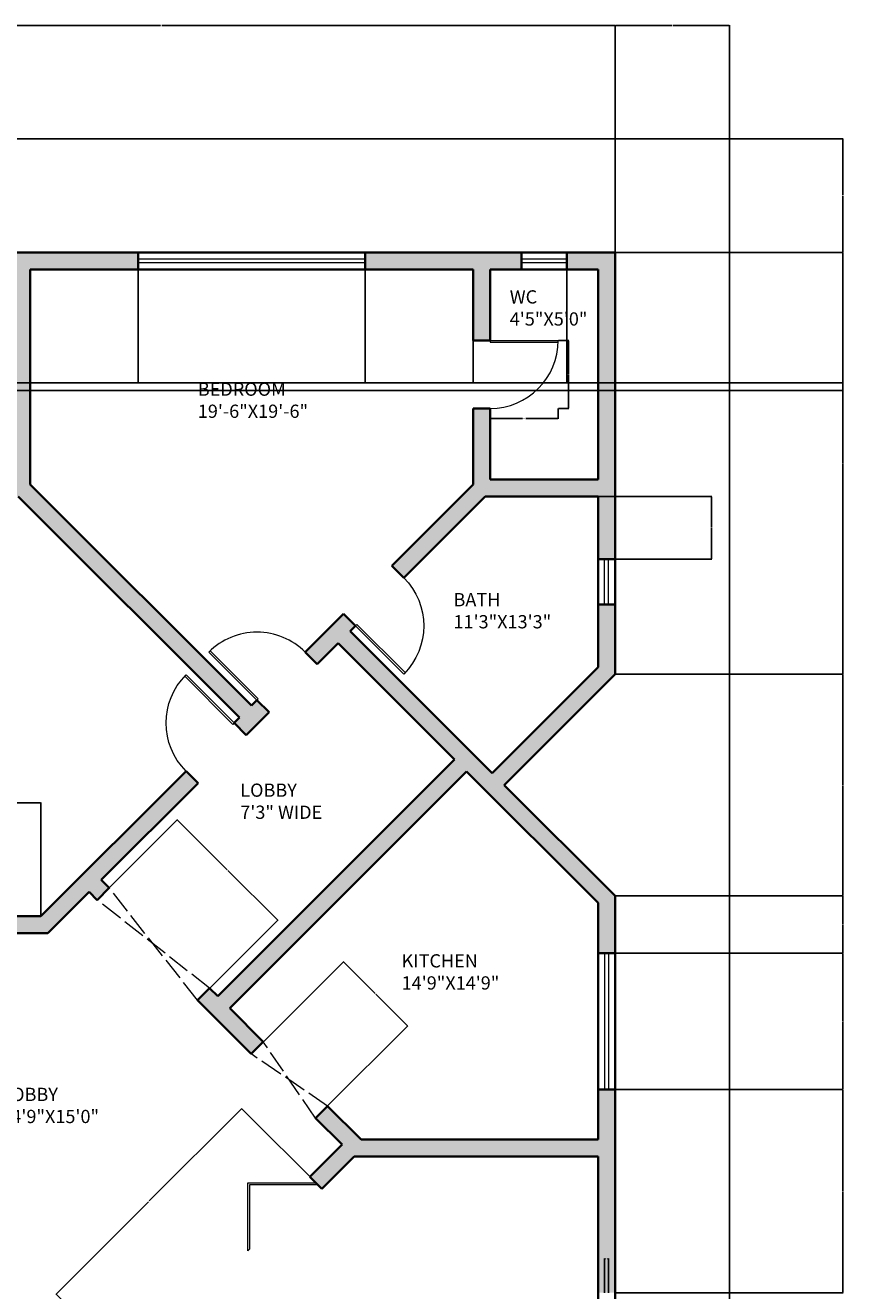
# Model space of a CAD drawing. Units: inches. Extents: x 1516 to 2236, y 3034 to 4235.
# Tile 3 of 3: x 1804 to 2236, y 3566 to 4235. Entities that reach past the tile are written whole.
import ezdxf

# ---------------------------------------------------------------- set-up
doc = ezdxf.new("R2010")
doc.units = ezdxf.units.IN
doc.linetypes.add('ACAD_ISO02W100', pattern=[15, 12, -3])
for name, color, linetype, lineweight in [('A-ANNO-DIMS', 2, 'Continuous', 18), ('A-AREA-IDEN', 7, 'Continuous', 18), ('A-DOOR', 3, 'Continuous', 18), ('A-GLAZ', 4, 'Continuous', 18), ('A-WALL', 7, 'Continuous', 35), ('A-WALL-OVHD', 8, 'ACAD_ISO02W100', 13), ('A-WALL-PATT', 252, 'Continuous', 13), ('C-PROP', 8, 'Continuous', 25)]:
    doc.layers.add(name, color=color, linetype=linetype, lineweight=lineweight)
doc.styles.get("Standard").update_dxf_attribs({"font": 'arial.ttf'})
doc.dimstyles.get("Standard").update_dxf_attribs({"dimtxt": 0.18, "dimasz": 0.18, "dimexe": 0.18, "dimexo": 0.0625, "dimgap": 0.09, "dimtad": 0, "dimtih": 1, "dimtoh": 1, "dimdec": 4, "dimzin": 0, "dimdsep": 46, "dimtxsty": 'Standard', "dimcen": 0.09, "dimadec": 0, "dimazin": 0, "dimtfac": 1, "dimtdec": 4, "dimtofl": 0, "dimtmove": 0, "dimatfit": 3, "dimfxl": 1, "dimtolj": 1, "dimtzin": 0, "dimarcsym": 0})

# ---------------------------------------------------------------- blocks, each defined once
blk = doc.blocks.new('DOOR-36IN-SWING')
for p, q in [((0, 36), (36, 36)), ((0, 36), (0, 35)), ((0, 35), (35.99, 35))]:
    blk.add_line(p, q)
blk.add_arc((0, 36), 36, 270, 0)
blk = doc.blocks.new('WIN-120IN-GLASS')
for p, q in [((120, 2), (0, 2)), ((120, 0), (0, 0))]:
    blk.add_line(p, q)
blk = doc.blocks.new('WIN-24IN-GLASS')
for p, q in [((24, 2), (0, 2)), ((24, 0), (0, 0))]:
    blk.add_line(p, q)
blk = doc.blocks.new('*D6')
at = {"layer": 'A-ANNO-DIMS', "color": 0, "lineweight": -2, "transparency": 16777216}
for p, q in [((2049.51, 4031.96), (2049.51, 4026.44)), ((2085.51, 4031.96), (2085.51, 4026.44)), ((2049.69, 4026.62), (2066.58, 4026.62)), ((2085.33, 4026.62), (2068.45, 4026.62))]:
    blk.add_line(p, q, dxfattribs=at)
at = {"layer": 'A-ANNO-DIMS', "color": 0, "transparency": 16777216}
for points in [[(2049.69, 4026.65), (2049.69, 4026.59), (2049.51, 4026.62)], [(2085.33, 4026.65), (2085.33, 4026.59), (2085.51, 4026.62)]]:
    blk.add_solid(points, dxfattribs=at)
at = {"layer": 'Defpoints', "color": 0, "transparency": 16777216}
for p in [(2049.51, 4032.02), (2085.51, 4032.02), (2085.51, 4026.62)]:
    blk.add_point(p, dxfattribs=at)
at = {"layer": 'A-ANNO-DIMS', "color": 0, "transparency": 16777216, "insert": (2067.51, 4026.62), "char_height": 0.18, "attachment_point": 5}
blk.add_mtext('\\A1;DOOR 36 TYP.', dxfattribs=at)
blk = doc.blocks.new('*D7')
at = {"layer": 'A-ANNO-DIMS', "color": 0, "lineweight": -2, "transparency": 16777216}
for p, q in [((2085.58, 4068.02), (2091.09, 4068.02)), ((2090.91, 4067.84), (2090.91, 4050.2)), ((2090.91, 4032.2), (2090.91, 4049.84)), ((2085.58, 4032.02), (2091.09, 4032.02))]:
    blk.add_line(p, q, dxfattribs=at)
at = {"layer": 'A-ANNO-DIMS', "color": 0, "transparency": 16777216}
for points in [[(2090.88, 4067.84), (2090.94, 4067.84), (2090.91, 4068.02)], [(2090.88, 4032.2), (2090.94, 4032.2), (2090.91, 4032.02)]]:
    blk.add_solid(points, dxfattribs=at)
at = {"layer": 'Defpoints', "color": 0, "transparency": 16777216}
for p in [(2085.51, 4068.02), (2090.91, 4068.02), (2085.51, 4032.02)]:
    blk.add_point(p, dxfattribs=at)
at = {"layer": 'A-ANNO-DIMS', "color": 0, "transparency": 16777216, "insert": (2090.91, 4050.02), "char_height": 0.18, "attachment_point": 5}
blk.add_mtext('\\A1;36 TYP.', dxfattribs=at)
blk = doc.blocks.new('*D13')
at = {"layer": 'A-ANNO-DIMS', "color": 0, "lineweight": -2, "transparency": 16777216}
for p, q in [((2110.01, 3564.47), (2110.01, 3582.59)), ((2110.19, 3582.41), (2110.55, 3582.41)), ((2111.83, 3582.41), (2111.47, 3582.41)), ((2112.01, 3564.47), (2112.01, 3582.59))]:
    blk.add_line(p, q, dxfattribs=at)
at = {"layer": 'A-ANNO-DIMS', "color": 0, "transparency": 16777216}
for points in [[(2110.19, 3582.44), (2110.19, 3582.38), (2110.01, 3582.41)], [(2111.83, 3582.44), (2111.83, 3582.38), (2112.01, 3582.41)]]:
    blk.add_solid(points, dxfattribs=at)
at = {"layer": 'Defpoints', "color": 0, "transparency": 16777216}
for p in [(2110.01, 3582.41), (2110.01, 3564.41), (2112.01, 3564.41)]:
    blk.add_point(p, dxfattribs=at)
at = {"layer": 'A-ANNO-DIMS', "color": 0, "transparency": 16777216, "insert": (2111.01, 3582.41), "char_height": 0.18, "attachment_point": 5}
blk.add_mtext('\\A1;2 TYP.', dxfattribs=at)
blk = doc.blocks.new('*D19')
at = {"layer": 'A-ANNO-DIMS', "color": 0, "lineweight": -2, "transparency": 16777216}
for p, q in [((1636.01, 4114.58), (1636.01, 4234.6)), ((1636.19, 4234.42), (1875.37, 4234.42)), ((2115.33, 4234.42), (1876.16, 4234.42)), ((2115.51, 4114.58), (2115.51, 4234.6))]:
    blk.add_line(p, q, dxfattribs=at)
at = {"layer": 'A-ANNO-DIMS', "color": 0, "transparency": 16777216}
for points in [[(1636.19, 4234.45), (1636.19, 4234.39), (1636.01, 4234.42)], [(2115.33, 4234.45), (2115.33, 4234.39), (2115.51, 4234.42)]]:
    blk.add_solid(points, dxfattribs=at)
at = {"layer": 'Defpoints', "color": 0, "transparency": 16777216}
for p in [(2115.51, 4234.42), (1636.01, 4114.52), (2115.51, 4114.52)]:
    blk.add_point(p, dxfattribs=at)
at = {"layer": 'A-ANNO-DIMS', "color": 0, "transparency": 16777216, "insert": (1875.76, 4234.42), "char_height": 0.18, "attachment_point": 5}
blk.add_mtext('\\A1;479.5', dxfattribs=at)
blk = doc.blocks.new('*D20')
at = {"layer": 'A-ANNO-DIMS', "color": 0, "lineweight": -2, "transparency": 16777216}
for p, q in [((2115.51, 4114.58), (2115.51, 4234.6)), ((2115.69, 4234.42), (2145.44, 4234.42)), ((2175.83, 4234.42), (2146.09, 4234.42)), ((2176.01, 4174.58), (2176.01, 4234.6))]:
    blk.add_line(p, q, dxfattribs=at)
at = {"layer": 'A-ANNO-DIMS', "color": 0, "transparency": 16777216}
for points in [[(2115.69, 4234.45), (2115.69, 4234.39), (2115.51, 4234.42)], [(2175.83, 4234.45), (2175.83, 4234.39), (2176.01, 4234.42)]]:
    blk.add_solid(points, dxfattribs=at)
at = {"layer": 'Defpoints', "color": 0, "transparency": 16777216}
for p in [(2176.01, 4234.42), (2176.01, 4174.52), (2115.51, 4114.52)]:
    blk.add_point(p, dxfattribs=at)
at = {"layer": 'A-ANNO-DIMS', "color": 0, "transparency": 16777216, "insert": (2145.76, 4234.42), "char_height": 0.18, "attachment_point": 5}
blk.add_mtext('\\A1;60.5', dxfattribs=at)
blk = doc.blocks.new('*D21')
at = {"layer": 'A-ANNO-DIMS', "color": 0, "lineweight": -2, "transparency": 16777216}
for p, q in [((2176.08, 4174.52), (2236.09, 4174.52)), ((2235.91, 4174.34), (2235.91, 4144.7)), ((2235.91, 4114.7), (2235.91, 4144.34)), ((2115.58, 4114.52), (2236.09, 4114.52))]:
    blk.add_line(p, q, dxfattribs=at)
at = {"layer": 'A-ANNO-DIMS', "color": 0, "transparency": 16777216}
for points in [[(2235.88, 4174.34), (2235.94, 4174.34), (2235.91, 4174.52)], [(2235.88, 4114.7), (2235.94, 4114.7), (2235.91, 4114.52)]]:
    blk.add_solid(points, dxfattribs=at)
at = {"layer": 'Defpoints', "color": 0, "transparency": 16777216}
for p in [(2176.01, 4174.52), (2235.91, 4174.52), (2115.51, 4114.52)]:
    blk.add_point(p, dxfattribs=at)
at = {"layer": 'A-ANNO-DIMS', "color": 0, "transparency": 16777216, "insert": (2235.91, 4144.52), "char_height": 0.18, "attachment_point": 5}
blk.add_mtext('\\A1;60', dxfattribs=at)
blk = doc.blocks.new('*D22')
at = {"layer": 'A-ANNO-DIMS', "color": 0, "lineweight": -2, "transparency": 16777216}
for p, q in [((2115.58, 4114.52), (2236.09, 4114.52)), ((2235.91, 4114.34), (2235.91, 4003.18)), ((2235.91, 3891.66), (2235.91, 4002.82)), ((2115.58, 3891.48), (2236.09, 3891.48))]:
    blk.add_line(p, q, dxfattribs=at)
at = {"layer": 'A-ANNO-DIMS', "color": 0, "transparency": 16777216}
for points in [[(2235.88, 4114.34), (2235.94, 4114.34), (2235.91, 4114.52)], [(2235.88, 3891.66), (2235.94, 3891.66), (2235.91, 3891.48)]]:
    blk.add_solid(points, dxfattribs=at)
at = {"layer": 'Defpoints', "color": 0, "transparency": 16777216}
for p in [(2115.51, 4114.52), (2235.91, 4114.52), (2115.51, 3891.48)]:
    blk.add_point(p, dxfattribs=at)
at = {"layer": 'A-ANNO-DIMS', "color": 0, "transparency": 16777216, "insert": (2235.91, 4003), "char_height": 0.18, "attachment_point": 5}
blk.add_mtext('\\A1;223.05', dxfattribs=at)
blk = doc.blocks.new('*D23')
at = {"layer": 'A-ANNO-DIMS', "color": 0, "lineweight": -2, "transparency": 16777216}
for p, q in [((2115.58, 3891.48), (2236.09, 3891.48)), ((2235.91, 3891.3), (2235.91, 3833.07)), ((2235.91, 3774.48), (2235.91, 3832.7)), ((2115.58, 3774.3), (2236.09, 3774.3))]:
    blk.add_line(p, q, dxfattribs=at)
at = {"layer": 'A-ANNO-DIMS', "color": 0, "transparency": 16777216}
for points in [[(2235.88, 3891.3), (2235.94, 3891.3), (2235.91, 3891.48)], [(2235.88, 3774.48), (2235.94, 3774.48), (2235.91, 3774.3)]]:
    blk.add_solid(points, dxfattribs=at)
at = {"layer": 'Defpoints', "color": 0, "transparency": 16777216}
for p in [(2115.51, 3891.48), (2235.91, 3891.48), (2115.51, 3774.3)]:
    blk.add_point(p, dxfattribs=at)
at = {"layer": 'A-ANNO-DIMS', "color": 0, "transparency": 16777216, "insert": (2235.91, 3832.89), "char_height": 0.18, "attachment_point": 5}
blk.add_mtext('\\A1;117.18', dxfattribs=at)
blk = doc.blocks.new('*D24')
at = {"layer": 'A-ANNO-DIMS', "color": 0, "lineweight": -2, "transparency": 16777216}
for p, q in [((2115.58, 3774.3), (2236.09, 3774.3)), ((2235.91, 3774.12), (2235.91, 3759.32)), ((2235.91, 3744.17), (2235.91, 3758.96)), ((2115.58, 3743.99), (2236.09, 3743.99))]:
    blk.add_line(p, q, dxfattribs=at)
at = {"layer": 'A-ANNO-DIMS', "color": 0, "transparency": 16777216}
for points in [[(2235.88, 3774.12), (2235.94, 3774.12), (2235.91, 3774.3)], [(2235.88, 3744.17), (2235.94, 3744.17), (2235.91, 3743.99)]]:
    blk.add_solid(points, dxfattribs=at)
at = {"layer": 'Defpoints', "color": 0, "transparency": 16777216}
for p in [(2115.51, 3774.3), (2235.91, 3774.3), (2115.51, 3743.99)]:
    blk.add_point(p, dxfattribs=at)
at = {"layer": 'A-ANNO-DIMS', "color": 0, "transparency": 16777216, "insert": (2235.91, 3759.14), "char_height": 0.18, "attachment_point": 5}
blk.add_mtext('\\A1;30.307', dxfattribs=at)
blk = doc.blocks.new('*D25')
at = {"layer": 'A-ANNO-DIMS', "color": 0, "lineweight": -2, "transparency": 16777216}
for p, q in [((2115.58, 3743.99), (2236.09, 3743.99)), ((2235.91, 3743.81), (2235.91, 3708.17)), ((2235.91, 3672.17), (2235.91, 3707.81)), ((2115.58, 3671.99), (2236.09, 3671.99))]:
    blk.add_line(p, q, dxfattribs=at)
at = {"layer": 'A-ANNO-DIMS', "color": 0, "transparency": 16777216}
for points in [[(2235.88, 3743.81), (2235.94, 3743.81), (2235.91, 3743.99)], [(2235.88, 3672.17), (2235.94, 3672.17), (2235.91, 3671.99)]]:
    blk.add_solid(points, dxfattribs=at)
at = {"layer": 'Defpoints', "color": 0, "transparency": 16777216}
for p in [(2115.51, 3743.99), (2235.91, 3743.99), (2115.51, 3671.99)]:
    blk.add_point(p, dxfattribs=at)
at = {"layer": 'A-ANNO-DIMS', "color": 0, "transparency": 16777216, "insert": (2235.91, 3707.99), "char_height": 0.18, "attachment_point": 5}
blk.add_mtext('\\A1;72', dxfattribs=at)
blk = doc.blocks.new('*D26')
at = {"layer": 'A-ANNO-DIMS', "color": 0, "lineweight": -2, "transparency": 16777216}
for p, q in [((2115.58, 3671.99), (2236.09, 3671.99)), ((2235.91, 3671.81), (2235.91, 3618.38)), ((2235.91, 3564.59), (2235.91, 3618.02)), ((2115.58, 3564.41), (2236.09, 3564.41))]:
    blk.add_line(p, q, dxfattribs=at)
at = {"layer": 'A-ANNO-DIMS', "color": 0, "transparency": 16777216}
for points in [[(2235.88, 3671.81), (2235.94, 3671.81), (2235.91, 3671.99)], [(2235.88, 3564.59), (2235.94, 3564.59), (2235.91, 3564.41)]]:
    blk.add_solid(points, dxfattribs=at)
at = {"layer": 'Defpoints', "color": 0, "transparency": 16777216}
for p in [(2115.51, 3671.99), (2235.91, 3671.99), (2115.51, 3564.41)]:
    blk.add_point(p, dxfattribs=at)
at = {"layer": 'A-ANNO-DIMS', "color": 0, "transparency": 16777216, "insert": (2235.91, 3618.2), "char_height": 0.18, "attachment_point": 5}
blk.add_mtext('\\A1;107.58', dxfattribs=at)
blk = doc.blocks.new('*D31')
at = {"layer": 'A-ANNO-DIMS', "color": 0, "lineweight": -2, "transparency": 16777216}
for p, q in [((1645.01, 3763.58), (1645.01, 3823.6)), ((1645.19, 3823.42), (1728.13, 3823.42)), ((1811.97, 3823.42), (1729.04, 3823.42)), ((1812.15, 3763.58), (1812.15, 3823.6))]:
    blk.add_line(p, q, dxfattribs=at)
at = {"layer": 'A-ANNO-DIMS', "color": 0, "transparency": 16777216}
for points in [[(1645.19, 3823.45), (1645.19, 3823.39), (1645.01, 3823.42)], [(1811.97, 3823.45), (1811.97, 3823.39), (1812.15, 3823.42)]]:
    blk.add_solid(points, dxfattribs=at)
at = {"layer": 'Defpoints', "color": 0, "transparency": 16777216}
for p in [(1812.15, 3823.42), (1645.01, 3763.52), (1812.15, 3763.52)]:
    blk.add_point(p, dxfattribs=at)
at = {"layer": 'A-ANNO-DIMS', "color": 0, "transparency": 16777216, "insert": (1728.58, 3823.42), "char_height": 0.18, "attachment_point": 5}
blk.add_mtext('\\A1;167.14', dxfattribs=at)
blk = doc.blocks.new('*D39')
at = {"layer": 'A-ANNO-DIMS', "color": 0, "lineweight": -2, "transparency": 16777216}
for p, q in [((1797.57679, 4045.522053), (2236.09429, 4045.522053)), ((1797.57679, 4041.522053), (2236.09429, 4041.522053)), ((2235.91429, 4045.342053), (2235.91429, 4043.702053)), ((2235.91429, 4041.702053), (2235.91429, 4043.342053))]:
    blk.add_line(p, q, dxfattribs=at)
at = {"layer": 'A-ANNO-DIMS', "color": 0, "transparency": 16777216}
for points in [[(2235.88429, 4045.342053), (2235.94429, 4045.342053), (2235.91429, 4045.522053)], [(2235.88429, 4041.702053), (2235.94429, 4041.702053), (2235.91429, 4041.522053)]]:
    blk.add_solid(points, dxfattribs=at)
at = {"layer": 'Defpoints', "color": 0, "transparency": 16777216}
for p in [(1797.51429, 4045.522053), (1797.51429, 4041.522053), (2235.91429, 4045.522053)]:
    blk.add_point(p, dxfattribs=at)
at = {"layer": 'A-ANNO-DIMS', "color": 0, "transparency": 16777216, "insert": (2235.91429, 4043.522053), "char_height": 0.18, "attachment_point": 5}
blk.add_mtext('\\A1;4', dxfattribs=at)
blk = doc.blocks.new('*D50')
at = {"layer": 'A-ANNO-DIMS', "color": 0, "lineweight": -2, "transparency": 16777216}
for p, q in [((1806.51, 4105.46), (1806.51, 4045.44)), ((1863.51, 4105.46), (1863.51, 4045.44)), ((1806.69, 4045.62), (1834.8, 4045.62)), ((1863.33, 4045.62), (1835.23, 4045.62))]:
    blk.add_line(p, q, dxfattribs=at)
at = {"layer": 'A-ANNO-DIMS', "color": 0, "transparency": 16777216}
for points in [[(1806.69, 4045.65), (1806.69, 4045.59), (1806.51, 4045.62)], [(1863.33, 4045.65), (1863.33, 4045.59), (1863.51, 4045.62)]]:
    blk.add_solid(points, dxfattribs=at)
at = {"layer": 'Defpoints', "color": 0, "transparency": 16777216}
for p in [(1806.51, 4105.52), (1863.51, 4105.52), (1806.51, 4045.62)]:
    blk.add_point(p, dxfattribs=at)
at = {"layer": 'A-ANNO-DIMS', "color": 0, "transparency": 16777216, "insert": (1835.01, 4045.62), "char_height": 0.18, "attachment_point": 5}
blk.add_mtext('\\A1;57', dxfattribs=at)
blk = doc.blocks.new('*D51')
at = {"layer": 'A-ANNO-DIMS', "color": 0, "lineweight": -2, "transparency": 16777216}
for p, q in [((1983.51, 4105.46), (1983.51, 4045.44)), ((2040.51, 4105.46), (2040.51, 4045.44)), ((1983.69, 4045.62), (2011.8, 4045.62)), ((2040.33, 4045.62), (2012.23, 4045.62))]:
    blk.add_line(p, q, dxfattribs=at)
at = {"layer": 'A-ANNO-DIMS', "color": 0, "transparency": 16777216}
for points in [[(1983.69, 4045.65), (1983.69, 4045.59), (1983.51, 4045.62)], [(2040.33, 4045.65), (2040.33, 4045.59), (2040.51, 4045.62)]]:
    blk.add_solid(points, dxfattribs=at)
at = {"layer": 'Defpoints', "color": 0, "transparency": 16777216}
for p in [(1983.51, 4105.52), (2040.51, 4105.52), (1983.51, 4045.62)]:
    blk.add_point(p, dxfattribs=at)
at = {"layer": 'A-ANNO-DIMS', "color": 0, "transparency": 16777216, "insert": (2012.01, 4045.62), "char_height": 0.18, "attachment_point": 5}
blk.add_mtext('\\A1;57', dxfattribs=at)
blk = doc.blocks.new('*D52')
at = {"layer": 'A-ANNO-DIMS', "color": 0, "lineweight": -2, "transparency": 16777216}
for p, q in [((2090.01, 4105.46), (2090.01, 4045.44)), ((2106.51, 4105.46), (2106.51, 4045.44)), ((2090.19, 4045.62), (2097.95, 4045.62)), ((2106.33, 4045.62), (2098.58, 4045.62))]:
    blk.add_line(p, q, dxfattribs=at)
at = {"layer": 'A-ANNO-DIMS', "color": 0, "transparency": 16777216}
for points in [[(2090.19, 4045.65), (2090.19, 4045.59), (2090.01, 4045.62)], [(2106.33, 4045.65), (2106.33, 4045.59), (2106.51, 4045.62)]]:
    blk.add_solid(points, dxfattribs=at)
at = {"layer": 'Defpoints', "color": 0, "transparency": 16777216}
for p in [(2090.01, 4105.52), (2106.51, 4105.52), (2090.01, 4045.62)]:
    blk.add_point(p, dxfattribs=at)
at = {"layer": 'A-ANNO-DIMS', "color": 0, "transparency": 16777216, "insert": (2098.26, 4045.62), "char_height": 0.18, "attachment_point": 5}
blk.add_mtext('\\A1;16.5', dxfattribs=at)
blk = doc.blocks.new('*D53')
at = {"layer": 'A-ANNO-DIMS', "color": 0, "lineweight": -2, "transparency": 16777216}
for p, q in [((2106.58, 3985.52), (2166.59, 3985.52)), ((2166.41, 3985.34), (2166.41, 3969.12)), ((2166.41, 3952.54), (2166.41, 3968.76)), ((2106.58, 3952.36), (2166.59, 3952.36))]:
    blk.add_line(p, q, dxfattribs=at)
at = {"layer": 'A-ANNO-DIMS', "color": 0, "transparency": 16777216}
for points in [[(2166.38, 3985.34), (2166.44, 3985.34), (2166.41, 3985.52)], [(2166.38, 3952.54), (2166.44, 3952.54), (2166.41, 3952.36)]]:
    blk.add_solid(points, dxfattribs=at)
at = {"layer": 'Defpoints', "color": 0, "transparency": 16777216}
for p in [(2106.51, 3985.52), (2106.51, 3952.36), (2166.41, 3952.36)]:
    blk.add_point(p, dxfattribs=at)
at = {"layer": 'A-ANNO-DIMS', "color": 0, "transparency": 16777216, "insert": (2166.41, 3968.94), "char_height": 0.18, "attachment_point": 5}
blk.add_mtext('\\A1;33.16', dxfattribs=at)
blk = doc.blocks.new('*D58')
at = {"layer": 'A-ANNO-DIMS', "color": 0, "lineweight": -2, "transparency": 16777216}
for p, q in [((1841.98, 3772.14), (1884.42, 3814.58)), ((1884.42, 3814.33), (1910.63, 3788.12)), ((1937.2, 3761.55), (1910.99, 3787.76)), ((1895.02, 3719.11), (1937.46, 3761.55))]:
    blk.add_line(p, q, dxfattribs=at)
at = {"layer": 'A-ANNO-DIMS', "color": 0, "transparency": 16777216}
for points in [[(1884.44, 3814.35), (1884.4, 3814.31), (1884.3, 3814.45)], [(1937.22, 3761.57), (1937.18, 3761.53), (1937.33, 3761.42)]]:
    blk.add_solid(points, dxfattribs=at)
at = {"layer": 'Defpoints', "color": 0, "transparency": 16777216}
for p in [(1841.94, 3772.1), (1937.33, 3761.42), (1894.97, 3719.07)]:
    blk.add_point(p, dxfattribs=at)
at = {"layer": 'A-ANNO-DIMS', "color": 0, "transparency": 16777216, "insert": (1910.81, 3787.94), "char_height": 0.18, "attachment_point": 5}
blk.add_mtext('\\A1;75', dxfattribs=at)
blk = doc.blocks.new('*D59')
at = {"layer": 'A-ANNO-DIMS', "color": 0, "lineweight": -2, "transparency": 16777216}
for p, q in [((1929.72, 3697.13), (1972.16, 3739.57)), ((1972.16, 3739.32), (1988.82, 3722.65)), ((2005.85, 3705.63), (1989.19, 3722.29)), ((1963.66, 3663.19), (2006.1, 3705.63))]:
    blk.add_line(p, q, dxfattribs=at)
at = {"layer": 'A-ANNO-DIMS', "color": 0, "transparency": 16777216}
for points in [[(1972.18, 3739.34), (1972.14, 3739.29), (1972.04, 3739.44)], [(2005.87, 3705.65), (2005.83, 3705.61), (2005.98, 3705.5)]]:
    blk.add_solid(points, dxfattribs=at)
at = {"layer": 'Defpoints', "color": 0, "transparency": 16777216}
for p in [(2005.98, 3705.5), (1929.68, 3697.09), (1963.62, 3663.15)]:
    blk.add_point(p, dxfattribs=at)
at = {"layer": 'A-ANNO-DIMS', "color": 0, "transparency": 16777216, "insert": (1989.01, 3722.47), "char_height": 0.18, "attachment_point": 5}
blk.add_mtext('\\A1;48', dxfattribs=at)
blk = doc.blocks.new('*D60')
at = {"layer": 'A-ANNO-DIMS', "color": 0, "lineweight": -2, "transparency": 16777216}
for p, q in [((1918.17, 3661.67), (1869.45, 3612.95)), ((1960.61, 3619.48), (1918.17, 3661.92)), ((1820.37, 3563.86), (1869.09, 3612.58)), ((1862.55, 3521.42), (1820.12, 3563.86))]:
    blk.add_line(p, q, dxfattribs=at)
at = {"layer": 'A-ANNO-DIMS', "color": 0, "transparency": 16777216}
for points in [[(1918.15, 3661.69), (1918.2, 3661.65), (1918.3, 3661.79)], [(1820.35, 3563.88), (1820.39, 3563.84), (1820.24, 3563.74)]]:
    blk.add_solid(points, dxfattribs=at)
at = {"layer": 'Defpoints', "color": 0, "transparency": 16777216}
for p in [(1918.3, 3661.79), (1960.66, 3619.44), (1862.6, 3521.38)]:
    blk.add_point(p, dxfattribs=at)
at = {"layer": 'A-ANNO-DIMS', "color": 0, "transparency": 16777216, "insert": (1869.27, 3612.77), "char_height": 0.18, "attachment_point": 5}
blk.add_mtext('\\A1;138.68', dxfattribs=at)

msp = doc.modelspace()

# ---------------------------------------------------------------- hatches: boundary and pattern name
at = {"layer": 'A-WALL-PATT'}
h = msp.add_hatch(color=256, dxfattribs=at)
h.dxf.hatch_style = 1
h.paths.add_polyline_path([(2115.5143, 3444.4097), (2106.5143, 3444.4097), (2106.5143, 3372.4097), (1977.6285, 3372.4097), (1845.6285, 3504.4097), (1862.599, 3521.3803), (1856.2351, 3527.7442), (1839.2645, 3510.7737), (1836.4361, 3513.6021), (1830.0721, 3507.2381), (1973.9005, 3363.4097), (2115.5143, 3363.4097)])
h.paths.add_polyline_path([(2115.5143, 3671.9887), (2106.5143, 3671.9887), (2106.5143, 3645.4097), (1981.3564, 3645.4097), (1963.6205, 3663.1456), (1957.2565, 3656.7817), (1971.2645, 3642.7737), (1954.2939, 3625.8031), (1960.6579, 3619.4391), (1977.6285, 3636.4097), (2106.5143, 3636.4097), (2106.5143, 3564.4097), (2115.5143, 3564.4097)])
h.paths.add_polyline_path([(1975.583, 3914.2268), (1978.4114, 3917.0552), (1972.0475, 3923.4192), (1951.7986, 3903.1703), (1958.1625, 3896.8063), (1969.219, 3907.8629), (2030.7373, 3846.3446), (1905.5794, 3721.1867), (1901.3368, 3725.4293), (1894.9728, 3719.0653), (1923.3154, 3690.7228), (1929.6793, 3697.0868), (1911.9434, 3714.8227), (2037.1013, 3839.9806), (2106.5143, 3770.5676), (2106.5143, 3743.9887), (2115.5143, 3743.9887), (2115.5143, 3774.2955), (2056.9238, 3832.886), (2115.5143, 3891.4765), (2115.5143, 3928.3632), (2106.5143, 3928.3632), (2106.5143, 3895.2044), (2050.5598, 3839.25)])
h.paths.add_polyline_path([(1806.5143, 3991.886), (1806.5143, 4105.5221), (1863.5143, 4105.5221), (1863.5143, 4114.5221), (1771.2643, 4114.5221), (1771.2643, 4105.5221), (1797.5143, 4105.5221), (1797.5143, 3994.5221), (1761.0143, 3994.5221), (1761.0143, 3985.5221), (1800.1503, 3985.5221), (1917.1503, 3868.5221), (1914.3219, 3865.6936), (1920.6859, 3859.3297), (1923.5143, 3862.1581), (1932.7067, 3871.3505), (1926.3427, 3877.7144), (1923.5143, 3874.886)])
h.paths.add_polyline_path([(1895.23, 3833.8738), (1888.8661, 3840.2378), (1812.1503, 3763.5221), (1645.0143, 3763.5221), (1645.0143, 3814.5221), (1636.0143, 3814.5221), (1636.0143, 3565.5221), (1771.7882, 3565.5221), (1779.1604, 3558.1498), (1785.5244, 3564.5138), (1775.5161, 3574.5221), (1645.0143, 3574.5221), (1645.0143, 3754.5221), (1815.8783, 3754.5221), (1837.6972, 3776.341), (1841.9398, 3772.0983), (1848.3038, 3778.4623), (1844.0611, 3782.7049)])
h.paths.add_polyline_path([(1645.0143, 3985.5221), (1725.0143, 3985.5221), (1725.0143, 3994.5221), (1721.0143, 3994.5221), (1721.0143, 3998.5221), (1717.0143, 3998.5221), (1717.0143, 3994.5221), (1645.0143, 3994.5221), (1645.0143, 4105.5221), (1669.0143, 4105.5221), (1669.0143, 4114.5221), (1636.0143, 4114.5221), (1636.0143, 3934.5221), (1645.0143, 3934.5221)])
h.paths.add_polyline_path([(1747.2643, 4114.5221), (1693.0143, 4114.5221), (1693.0143, 4105.5221), (1717.0143, 4105.5221), (1717.0143, 4028.5221), (1721.0143, 4028.5221), (1721.0143, 4041.5221), (1725.0143, 4041.5221), (1725.0143, 4045.5221), (1721.0143, 4045.5221), (1721.0143, 4105.5221), (1747.2643, 4105.5221)])
h.paths.add_polyline_path([(2066.0143, 4114.5221), (1983.5143, 4114.5221), (1983.5143, 4105.5221), (2040.5143, 4105.5221), (2040.5143, 4068.0221), (2049.5143, 4068.0221), (2049.5143, 4105.5221), (2066.0143, 4105.5221)])
h.paths.add_polyline_path([(2115.5143, 4114.5221), (2090.0143, 4114.5221), (2090.0143, 4105.5221), (2106.5143, 4105.5221), (2106.5143, 3994.5221), (2049.5143, 3994.5221), (2049.5143, 4032.0221), (2040.5143, 4032.0221), (2040.5143, 3991.886), (1997.5033, 3948.875), (2003.8673, 3942.5111), (2046.8783, 3985.5221), (2106.5143, 3985.5221), (2106.5143, 3952.3632), (2115.5143, 3952.3632)])
h.paths.add_polyline_path([(1789.2236, 3395.8151), (1636.0143, 3395.8151), (1636.0143, 3386.8151), (1785.4957, 3386.8151), (1891.4008, 3280.91), (1897.7648, 3287.2739)])

# ---------------------------------------------------------------- linework, layer by layer
at = {"layer": 'A-DOOR'}
for p, q in [((1921.4759, 3586.6211), (1921.4759, 3622.6211)), ((1921.4759, 3622.6211), (1957.4759, 3622.6211)), ((1922.4759, 3587.6211), (1922.4759, 3621.6211)), ((1922.4759, 3621.6211), (1958.4759, 3621.6211)), ((1922.4759, 3587.6211), (1921.4759, 3586.6211))]:
    msp.add_line(p, q, dxfattribs=at)
at = {"layer": 'A-GLAZ'}
for p, q in [((2110.0143, 3743.9887), (2110.0143, 3671.9887)), ((2112.0143, 3743.9887), (2112.0143, 3671.9887))]:
    msp.add_line(p, q, dxfattribs=at)
at = {"layer": 'A-WALL'}
for p, q in [((1636.0143, 4114.5221), (2115.5143, 4114.5221)), ((1863.5143, 4105.5221), (1863.5143, 4114.5221)), ((1983.5143, 4105.5221), (1983.5143, 4114.5221)), ((2066.0143, 4105.5221), (2066.0143, 4114.5221)), ((2090.0143, 4105.5221), (2090.0143, 4114.5221)), ((2115.5143, 4114.5221), (2115.5143, 3891.4765)), ((1806.5143, 4105.5221), (1806.5143, 3991.886)), ((1806.5143, 4105.5221), (2040.5143, 4105.5221)), ((2040.5143, 4105.5221), (2040.5143, 4068.0221)), ((2049.5143, 4105.5221), (2049.5143, 4068.0221)), ((2049.5143, 4105.5221), (2106.5143, 4105.5221)), ((2106.5143, 4105.5221), (2106.5143, 3994.5221)), ((2049.5143, 4068.0221), (2040.5143, 4068.0221)), ((2049.5143, 4032.0221), (2040.5143, 4032.0221)), ((2040.5143, 4032.0221), (2040.5143, 3991.886)), ((2049.5143, 4032.0221), (2049.5143, 3994.5221)), ((2049.5143, 3994.5221), (2106.5143, 3994.5221)), ((1806.5143, 3991.886), (1923.5143, 3874.886)), ((2040.5143, 3991.886), (1997.5033, 3948.875)), ((1800.1503, 3985.5221), (1917.1503, 3868.5221)), ((2046.8783, 3985.5221), (2003.8673, 3942.5111)), ((2046.8783, 3985.5221), (2106.5143, 3985.5221)), ((2106.5143, 3985.5221), (2106.5143, 3895.2044)), ((1997.5033, 3948.875), (2003.8673, 3942.5111)), ((2106.5143, 3952.3632), (2115.5143, 3952.3632)), ((2106.5143, 3928.3632), (2115.5143, 3928.3632)), ((1972.0475, 3923.4192), (1951.7986, 3903.1703)), ((1972.0475, 3923.4192), (1978.4114, 3917.0552)), ((1978.4114, 3917.0552), (1975.583, 3914.2268)), ((1975.583, 3914.2268), (2050.5598, 3839.25)), ((1969.219, 3907.8629), (1958.1625, 3896.8063)), ((1969.219, 3907.8629), (2030.7373, 3846.3446)), ((1951.7986, 3903.1703), (1958.1625, 3896.8063)), ((2106.5143, 3895.2044), (2050.5598, 3839.25)), ((2115.5143, 3891.4765), (2056.9238, 3832.886)), ((1926.3427, 3877.7144), (1923.5143, 3874.886)), ((1926.3427, 3877.7144), (1932.7067, 3871.3505)), ((1914.3219, 3865.6936), (1917.1503, 3868.5221)), ((1932.7067, 3871.3505), (1923.5143, 3862.1581)), ((1914.3219, 3865.6936), (1920.6859, 3859.3297)), ((1920.6859, 3859.3297), (1923.5143, 3862.1581)), ((1905.5794, 3721.1867), (2030.7373, 3846.3446)), ((1812.1503, 3763.5221), (1888.8661, 3840.2378)), ((1844.0611, 3782.7049), (1895.23, 3833.8738)), ((1888.8661, 3840.2378), (1895.23, 3833.8738)), ((1911.9434, 3714.8227), (2037.1013, 3839.9806)), ((2037.1013, 3839.9806), (2106.5143, 3770.5676)), ((2056.9238, 3832.886), (2115.5143, 3774.2955)), ((1844.0611, 3782.7049), (1848.3038, 3778.4623)), ((1815.8783, 3754.5221), (1837.6972, 3776.341)), ((1837.6972, 3776.341), (1841.9398, 3772.0983)), ((1841.9398, 3772.0983), (1848.3038, 3778.4623)), ((2115.5143, 3774.2955), (2115.5143, 3363.4097)), ((2106.5143, 3770.5676), (2106.5143, 3645.4097)), ((1645.0143, 3763.5221), (1812.1503, 3763.5221)), ((1645.0143, 3754.5221), (1815.8783, 3754.5221)), ((2106.5143, 3743.9887), (2115.5143, 3743.9887)), ((1894.9728, 3719.0653), (1901.3368, 3725.4293)), ((1901.3368, 3725.4293), (1905.5794, 3721.1867)), ((1894.9728, 3719.0653), (1923.3154, 3690.7228)), ((1911.9434, 3714.8227), (1929.6793, 3697.0868)), ((1929.6793, 3697.0868), (1923.3154, 3690.7228)), ((2106.5143, 3671.9887), (2115.5143, 3671.9887)), ((1963.6205, 3663.1456), (1957.2565, 3656.7817)), ((1963.6205, 3663.1456), (1981.3564, 3645.4097)), ((1957.2565, 3656.7817), (1971.2645, 3642.7737)), ((1954.2939, 3625.8031), (1971.2645, 3642.7737)), ((1981.3564, 3645.4097), (2106.5143, 3645.4097)), ((1960.6579, 3619.4391), (1977.6285, 3636.4097)), ((1977.6285, 3636.4097), (2106.5143, 3636.4097)), ((2106.5143, 3636.4097), (2106.5143, 3372.4097)), ((1954.2939, 3625.8031), (1960.6579, 3619.4391))]:
    msp.add_line(p, q, dxfattribs=at)
at = {"layer": 'A-WALL-OVHD'}
for p, q in [((1894.9728, 3719.0653), (1848.3038, 3778.4623)), ((1901.3368, 3725.4293), (1841.9398, 3772.0983)), ((1957.2565, 3656.7817), (1929.6793, 3697.0868)), ((1963.6205, 3663.1456), (1923.3154, 3690.7228))]:
    msp.add_line(p, q, dxfattribs=at)
at = {"layer": 'C-PROP'}
for p, q in [((1576.0143, 4174.5221), (2176.0143, 4174.5221)), ((2176.0143, 4174.5221), (2176.0143, 3094.5221))]:
    msp.add_line(p, q, dxfattribs=at)

# ---------------------------------------------------------------- block references
at = {"layer": 'A-DOOR'}
msp.add_blockref('DOOR-36IN-SWING', (2049.5143, 4032.0221), dxfattribs=at)
at = {"layer": 'A-DOOR', "extrusion": (0, 0, -1), "zscale": -1}
for p, rotation in [((-2003.8673, 3942.5111), 224.9999999999896), ((-1888.8661, 3840.2378), 45.00000000000024)]:
    msp.add_blockref('DOOR-36IN-SWING', p, dxfattribs=dict(at, rotation=rotation))
at = {"layer": 'A-DOOR', "rotation": 135.0000000000014}
msp.add_blockref('DOOR-36IN-SWING', (1951.7986, 3903.1703), dxfattribs=at)
at = {"layer": 'A-GLAZ'}
for name, p in [('WIN-120IN-GLASS', (1863.5143, 4109.0221)), ('WIN-24IN-GLASS', (2066.0143, 4109.0221))]:
    msp.add_blockref(name, p, dxfattribs=at)
at = {"layer": 'A-GLAZ', "rotation": 270}
msp.add_blockref('WIN-24IN-GLASS', (2110.0143, 3952.3632), dxfattribs=at)

# ---------------------------------------------------------------- texts
at = {"layer": 'A-AREA-IDEN', "char_height": 7, "attachment_point": 1}
for s, insert in [('WC\\P4\'5"X5\'0"', (2059.8878, 4094.4995)), ('BEDROOM\\P19\'-6"X19\'-6"', (1895.0812, 4045.702)), ('BATH\\P11\'3"X13\'3"', (2030.1572, 3934.3924)), ('LOBBY\\P7\'3" WIDE', (1917.5181, 3833.6783)), ('KITCHEN\\P14\'9"X14\'9"', (2002.7615, 3743.4274)), ('LOBBY\\P24\'9"X15\'0"', (1791.2759, 3672.8127))]:
    msp.add_mtext_dynamic_manual_height_columns(s, width=47.692137, gutter_width=12.5, heights=[0], dxfattribs=dict(at, insert=insert))

# ---------------------------------------------------------------- dimensions: what is measured, and where the dimension line sits
at = {"layer": 'A-ANNO-DIMS'}
for base, p1, p2, override, picture, middle in [((2115.5143, 4234.4221), (1636.0143, 4114.5221), (2115.5143, 4114.5221), {"dimdec": 1, "dimlfac": 1, "dimrnd": 0, "dimzin": 0, "dimdsep": 46, "dimlunit": 2}, '*D19', (1875.7643, 4234.4221)), ((2176.0143, 4234.4221), (2115.5143, 4114.5221), (2176.0143, 4174.5221), {"dimdec": 1, "dimlfac": 1, "dimrnd": 0, "dimzin": 0, "dimdsep": 46, "dimlunit": 2}, '*D20', (2145.7643, 4234.4221)), ((1812.1503, 3823.4221), (1645.0143, 3763.5221), (1812.1503, 3763.5221), {"dimdec": 2, "dimlfac": 1, "dimrnd": 0, "dimzin": 0, "dimdsep": 46, "dimlunit": 2}, '*D31', (1728.5823, 3823.4221))]:
    dim = msp.add_linear_dim(base=base, p1=p1, p2=p2, dimstyle='Standard', override=override, dxfattribs=at)
    dim.commit()
    dim.dimension.update_dxf_attribs({"geometry": picture, "text_midpoint": middle})
for base, p1, p2, angle, override, picture, middle in [((2235.9143, 4174.5221), (2115.5143, 4114.5221), (2176.0143, 4174.5221), 90, {"dimdec": 0, "dimlfac": 1, "dimrnd": 0, "dimzin": 0, "dimdsep": 46, "dimlunit": 2}, '*D21', (2235.9143, 4144.5221)), ((2235.9143, 4114.5221), (2115.5143, 3891.4765), (2115.5143, 4114.5221), 90, {"dimdec": 2, "dimlfac": 1, "dimrnd": 0, "dimzin": 0, "dimdsep": 46, "dimlunit": 2}, '*D22', (2235.9143, 4002.9993)), ((1806.5143, 4045.6221), (1863.5143, 4105.5221), (1806.5143, 4105.5221), 180, {"dimdec": 0, "dimlfac": 1, "dimrnd": 0, "dimzin": 0, "dimdsep": 46, "dimlunit": 2}, '*D50', (1835.0143, 4045.6221)), ((1983.5143, 4045.6221), (2040.5143, 4105.5221), (1983.5143, 4105.5221), 180, {"dimdec": 0, "dimlfac": 1, "dimrnd": 0, "dimzin": 0, "dimdsep": 46, "dimlunit": 2}, '*D51', (2012.0143, 4045.6221)), ((2090.0143, 4045.6221), (2106.5143, 4105.5221), (2090.0143, 4105.5221), 180, {"dimdec": 1, "dimlfac": 1, "dimrnd": 0, "dimzin": 0, "dimdsep": 46, "dimlunit": 2}, '*D52', (2098.2643, 4045.6221)), ((2235.9143, 4045.5221), (1797.5143, 4041.5221), (1797.5143, 4045.5221), 90, {"dimdec": 0, "dimlfac": 1, "dimrnd": 0, "dimzin": 0, "dimdsep": 46, "dimlunit": 2}, '*D39', (2235.9143, 4043.5221)), ((2166.4143, 3952.3632), (2106.5143, 3985.5221), (2106.5143, 3952.3632), 270, {"dimdec": 2, "dimlfac": 1, "dimrnd": 0, "dimzin": 0, "dimdsep": 46, "dimlunit": 2}, '*D53', (2166.4143, 3968.9426)), ((2235.9143, 3891.4765), (2115.5143, 3774.2955), (2115.5143, 3891.4765), 90, {"dimdec": 2, "dimlfac": 1, "dimrnd": 0, "dimzin": 0, "dimdsep": 46, "dimlunit": 2}, '*D23', (2235.9143, 3832.886)), ((1937.3285, 3761.421), (1841.9398, 3772.0983), (1894.9728, 3719.0653), 315, {"dimdec": 0, "dimlfac": 1, "dimrnd": 0, "dimzin": 0, "dimdsep": 46, "dimlunit": 2}, '*D58', (1910.812, 3787.9375)), ((2235.9143, 3774.2955), (2115.5143, 3743.9887), (2115.5143, 3774.2955), 90, {"dimdec": 3, "dimlfac": 1, "dimrnd": 0, "dimzin": 0, "dimdsep": 46, "dimlunit": 2}, '*D24', (2235.9143, 3759.1421)), ((2235.9143, 3743.9887), (2115.5143, 3671.9887), (2115.5143, 3743.9887), 90, {"dimdec": 0, "dimlfac": 1, "dimrnd": 0, "dimzin": 0, "dimdsep": 46, "dimlunit": 2}, '*D25', (2235.9143, 3707.9887)), ((2005.9762, 3705.5013), (1929.6793, 3697.0868), (1963.6205, 3663.1456), 315, {"dimdec": 0, "dimlfac": 1, "dimrnd": 0, "dimzin": 0, "dimdsep": 46, "dimlunit": 2}, '*D59', (1989.0056, 3722.4719)), ((2235.9143, 3671.9887), (2115.5143, 3564.4097), (2115.5143, 3671.9887), 90, {"dimdec": 2, "dimlfac": 1, "dimrnd": 0, "dimzin": 0, "dimdsep": 46, "dimlunit": 2}, '*D26', (2235.9143, 3618.1992)), ((1918.3022, 3661.7948), (1862.599, 3521.3803), (1960.6579, 3619.4391), 45, {"dimdec": 2, "dimlfac": 1, "dimrnd": 0, "dimzin": 0, "dimdsep": 46, "dimlunit": 2}, '*D60', (1869.2728, 3612.7654))]:
    dim = msp.add_linear_dim(base=base, p1=p1, p2=p2, angle=angle, dimstyle='Standard', override=override, dxfattribs=at)
    dim.commit()
    dim.dimension.update_dxf_attribs({"geometry": picture, "text_midpoint": middle})
for base, p1, p2, angle, picture, middle in [((2090.9143, 4068.0221), (2085.5143, 4032.0221), (2085.5143, 4068.0221), 90, '*D7', (2090.9143, 4050.0221)), ((2110.0143, 3582.4097), (2112.0143, 3564.4097), (2110.0143, 3564.4097), 180, '*D13', (2111.0143, 3582.4097))]:
    dim = msp.add_linear_dim(base=base, p1=p1, p2=p2, angle=angle, text='<> TYP.', dimstyle='Standard', override={"dimdec": 0, "dimlfac": 1, "dimrnd": 0, "dimzin": 0, "dimdsep": 46, "dimlunit": 2}, dxfattribs=at)
    dim.commit()
    dim.dimension.update_dxf_attribs({"geometry": picture, "text_midpoint": middle})
dim = msp.add_linear_dim(base=(2085.5143, 4026.6221), p1=(2049.5143, 4032.0221), p2=(2085.5143, 4032.0221), text='DOOR <> TYP.', dimstyle='Standard', override={"dimdec": 0, "dimlfac": 1, "dimrnd": 0, "dimzin": 0, "dimdsep": 46, "dimlunit": 2}, dxfattribs=at)
dim.commit()
dim.dimension.update_dxf_attribs({"geometry": '*D6', "text_midpoint": (2067.5143, 4026.6221)})

doc.saveas('drawing.dxf')
